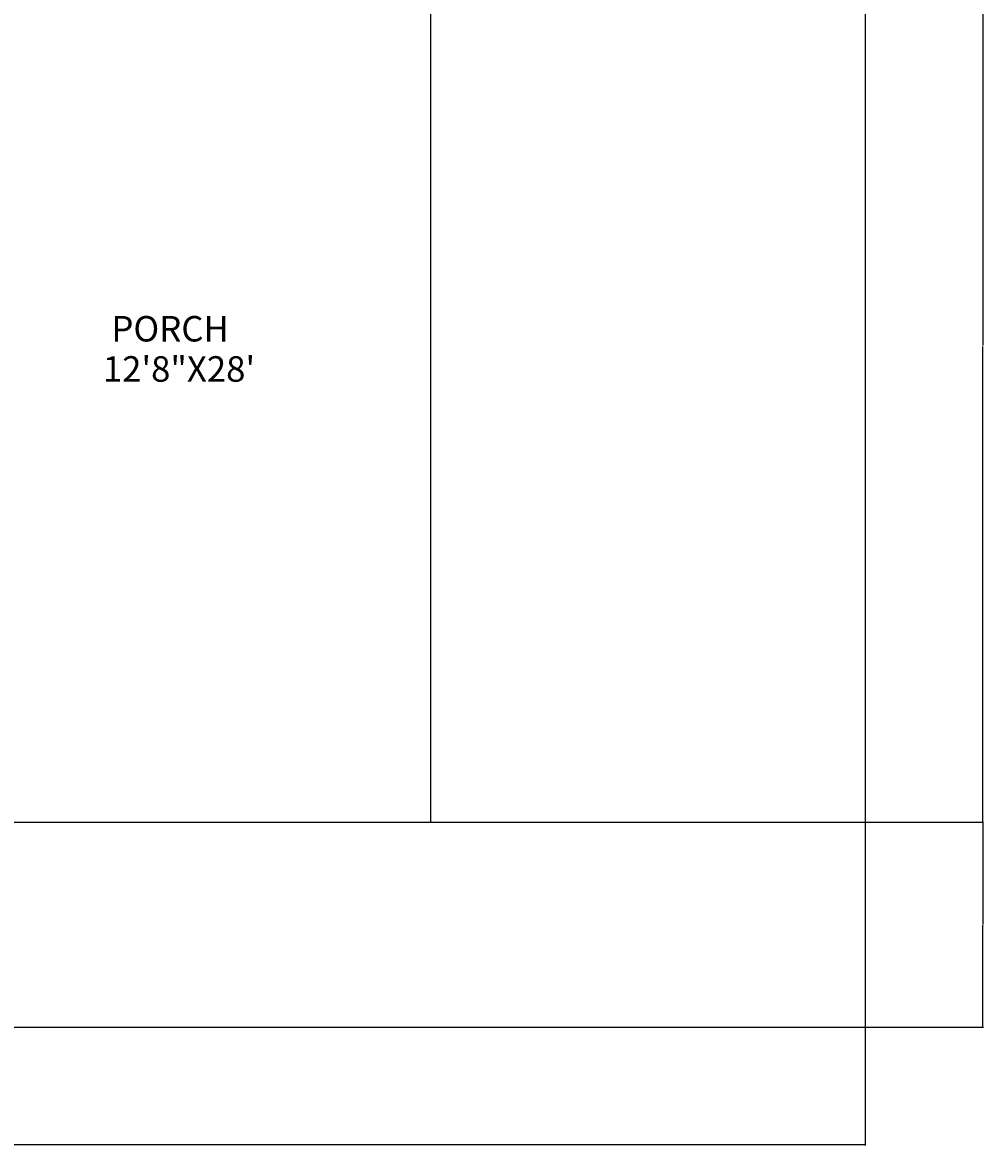
# Model space of a CAD drawing. Units: feet. Extents: x 2032 to 2763, y 1402 to 2145.
# Tile 2 of 6: x 2482 to 2763, y 1402 to 1731. Entities that reach past the tile are written whole.
import ezdxf

# ---------------------------------------------------------------- set-up
doc = ezdxf.new("R2010")
doc.units = ezdxf.units.FT
for name, color, linetype, lineweight in [('A-ANNO-DIMS', 2, 'Continuous', 18), ('A-AREA-IDEN', 7, 'Continuous', 25), ('A-FLOR', 7, 'Continuous', 25), ('C-PROP', 8, 'Continuous', 25)]:
    doc.layers.add(name, color=color, linetype=linetype, lineweight=lineweight)
doc.styles.get("Standard").update_dxf_attribs({"font": 'arial.ttf'})
doc.dimstyles.get("Standard").update_dxf_attribs({"dimtxt": 0.18, "dimasz": 0.18, "dimexe": 0.18, "dimexo": 0.0625, "dimgap": 0.09, "dimtad": 0, "dimtih": 1, "dimtoh": 1, "dimdec": 4, "dimzin": 0, "dimdsep": 46, "dimtxsty": 'Standard', "dimcen": 0.09, "dimadec": 0, "dimazin": 0, "dimtfac": 1, "dimtdec": 4, "dimtofl": 0, "dimtmove": 0, "dimatfit": 3, "dimfxl": 1, "dimtolj": 1, "dimtzin": 0, "dimarcsym": 0})

# ---------------------------------------------------------------- blocks, each defined once
blk = doc.blocks.new('*D33')
at = {"layer": 'A-ANNO-DIMS', "color": 0, "lineweight": -2, "transparency": 16777216}
for p, q in [((2067.31, 1436.55), (2067.31, 1401.93)), ((2728.31, 1436.55), (2728.31, 1401.93)), ((2067.49, 1402.11), (2397.54, 1402.11)), ((2728.13, 1402.11), (2398.09, 1402.11))]:
    blk.add_line(p, q, dxfattribs=at)
at = {"layer": 'A-ANNO-DIMS', "color": 0, "transparency": 16777216}
for points in [[(2067.49, 1402.14), (2067.49, 1402.08), (2067.31, 1402.11)], [(2728.13, 1402.14), (2728.13, 1402.08), (2728.31, 1402.11)]]:
    blk.add_solid(points, dxfattribs=at)
at = {"layer": 'Defpoints', "color": 0, "transparency": 16777216}
for p in [(2067.31, 1436.61), (2728.31, 1436.61), (2728.31, 1402.11)]:
    blk.add_point(p, dxfattribs=at)
at = {"layer": 'A-ANNO-DIMS', "color": 0, "transparency": 16777216, "insert": (2397.81, 1402.11), "char_height": 0.18, "attachment_point": 5}
blk.add_mtext('\\A1;661', dxfattribs=at)
blk = doc.blocks.new('*D47')
at = {"layer": 'A-ANNO-DIMS', "color": 0, "lineweight": -2, "transparency": 16777216}
for p, q in [((2601.22, 1496.61), (2762.99, 1496.61)), ((2762.81, 1496.43), (2762.81, 1466.79)), ((2762.81, 1436.79), (2762.81, 1466.43)), ((2728.38, 1436.61), (2762.99, 1436.61))]:
    blk.add_line(p, q, dxfattribs=at)
at = {"layer": 'A-ANNO-DIMS', "color": 0, "transparency": 16777216}
for points in [[(2762.78, 1496.43), (2762.84, 1496.43), (2762.81, 1496.61)], [(2762.78, 1436.79), (2762.84, 1436.79), (2762.81, 1436.61)]]:
    blk.add_solid(points, dxfattribs=at)
at = {"layer": 'Defpoints', "color": 0, "transparency": 16777216}
for p in [(2601.16, 1496.61), (2762.81, 1496.61), (2728.31, 1436.61)]:
    blk.add_point(p, dxfattribs=at)
at = {"layer": 'A-ANNO-DIMS', "color": 0, "transparency": 16777216, "insert": (2762.81, 1466.61), "char_height": 0.18, "attachment_point": 5}
blk.add_mtext('\\A1;60', dxfattribs=at)
blk = doc.blocks.new('*D48')
at = {"layer": 'A-ANNO-DIMS', "color": 0, "lineweight": -2, "transparency": 16777216}
for p, q in [((2601.22, 1775.61), (2762.99, 1775.61)), ((2762.81, 1775.43), (2762.81, 1636.29)), ((2762.81, 1496.79), (2762.81, 1635.93)), ((2601.22, 1496.61), (2762.99, 1496.61))]:
    blk.add_line(p, q, dxfattribs=at)
at = {"layer": 'A-ANNO-DIMS', "color": 0, "transparency": 16777216}
for points in [[(2762.78, 1775.43), (2762.84, 1775.43), (2762.81, 1775.61)], [(2762.78, 1496.79), (2762.84, 1496.79), (2762.81, 1496.61)]]:
    blk.add_solid(points, dxfattribs=at)
at = {"layer": 'Defpoints', "color": 0, "transparency": 16777216}
for p in [(2601.16, 1775.61), (2762.81, 1775.61), (2601.16, 1496.61)]:
    blk.add_point(p, dxfattribs=at)
at = {"layer": 'A-ANNO-DIMS', "color": 0, "transparency": 16777216, "insert": (2762.81, 1636.11), "char_height": 0.18, "attachment_point": 5}
blk.add_mtext('\\A1;279', dxfattribs=at)

msp = doc.modelspace()

# ---------------------------------------------------------------- linework, layer by layer
at = {"layer": 'A-FLOR'}
for p, q in [((2601.1579, 1496.6131), (2601.1579, 1775.6131)), ((2127.3136, 1496.6131), (2601.1579, 1496.6131))]:
    msp.add_line(p, q, dxfattribs=at)
at = {"layer": 'C-PROP'}
for p, q in [((2728.3136, 2110.6131), (2728.3136, 1496.6131)), ((2728.3136, 1496.6131), (2728.3136, 1436.6131)), ((2067.3136, 1436.6131), (2728.3136, 1436.6131))]:
    msp.add_line(p, q, dxfattribs=at)

# ---------------------------------------------------------------- texts
at = {"layer": 'A-AREA-IDEN'}
for s, p in [('PORCH', (2507.6287, 1637.3419)), ('12\'8"X28\'', (2505.1178, 1625.5707))]:
    msp.add_text(s, height=7.46821, dxfattribs=at).set_placement(p)

# ---------------------------------------------------------------- dimensions: what is measured, and where the dimension line sits
at = {"layer": 'A-ANNO-DIMS'}
for base, p1, p2, picture, middle in [((2762.8136, 1775.6131), (2601.1579, 1496.6131), (2601.1579, 1775.6131), '*D48', (2762.8136, 1636.1131)), ((2762.8136, 1496.6131), (2728.3136, 1436.6131), (2601.1579, 1496.6131), '*D47', (2762.8136, 1466.6131))]:
    dim = msp.add_linear_dim(base=base, p1=p1, p2=p2, angle=90, dimstyle='Standard', override={"dimdec": 0, "dimlfac": 1, "dimrnd": 0, "dimzin": 0, "dimdsep": 46, "dimlunit": 2}, dxfattribs=at)
    dim.commit()
    dim.dimension.update_dxf_attribs({"geometry": picture, "text_midpoint": middle})
dim = msp.add_linear_dim(base=(2728.3136, 1402.1131), p1=(2067.3136, 1436.6131), p2=(2728.3136, 1436.6131), dimstyle='Standard', override={"dimdec": 0, "dimlfac": 1, "dimrnd": 0, "dimzin": 0, "dimdsep": 46, "dimlunit": 2}, dxfattribs=at)
dim.commit()
dim.dimension.update_dxf_attribs({"geometry": '*D33', "text_midpoint": (2397.8136, 1402.1131)})

doc.saveas('drawing.dxf')
